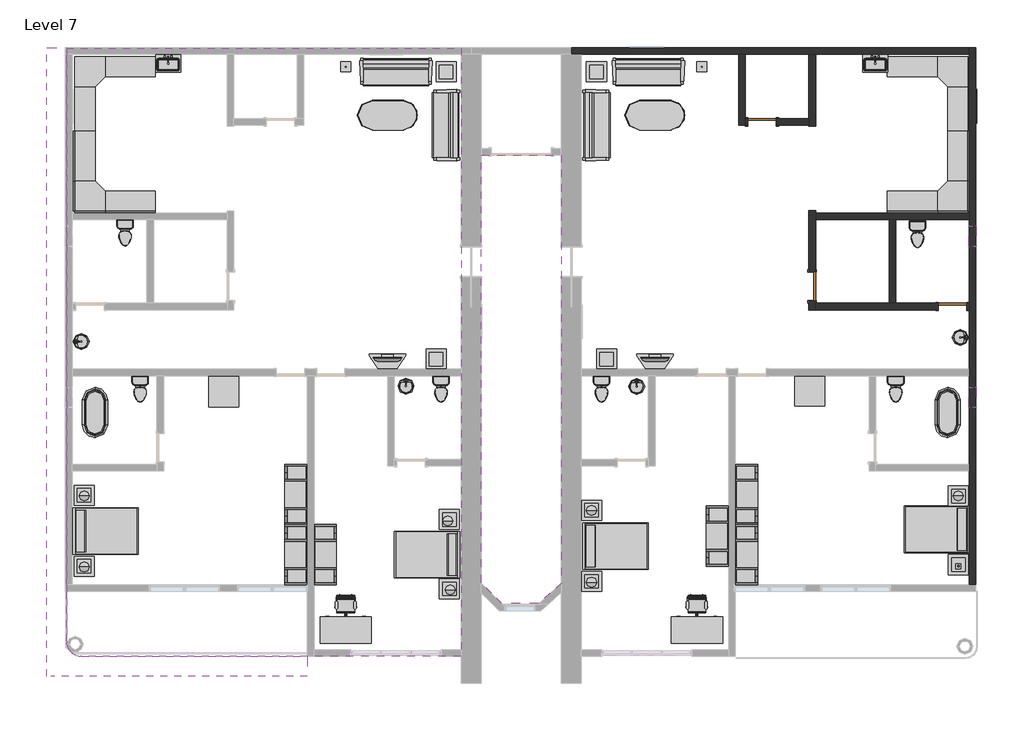
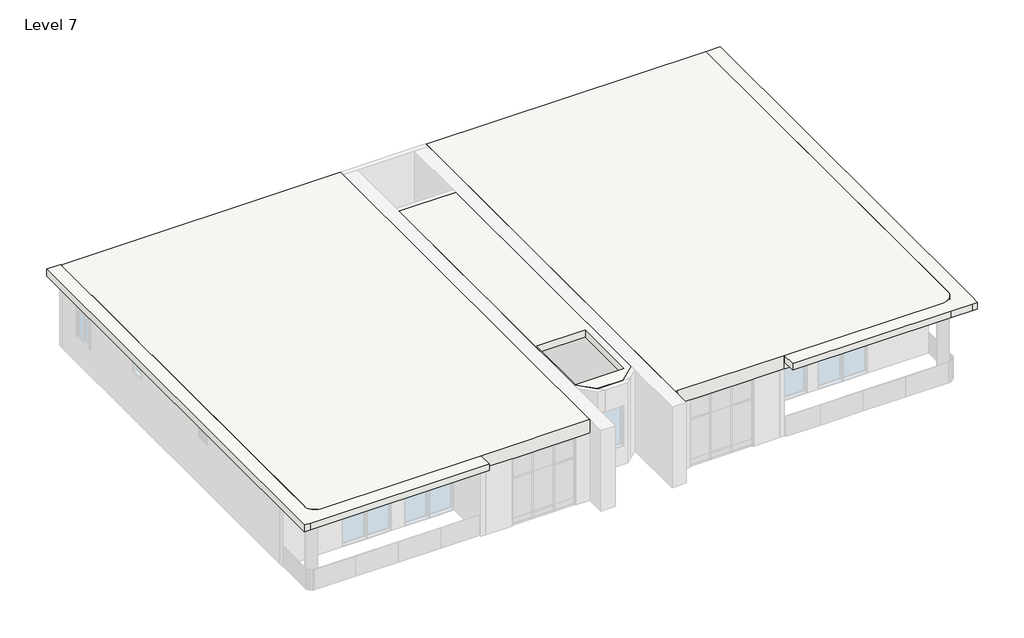
# One storey, part 3 of 3: 42 furniture elements, 14 flow terminals, 10 light fixtures, 9 walls, 3 doors, 3 slabs, 3 windows.
"""IFC4 building model written with IfcOpenShell, lengths in millimetres."""

from ifc_helpers import new_model, si_unit, point, frame, frame_2d, origin, place, context, project, spatial, polyline, circle_curve, trimmed, segment, composite_curve, outline, extrude, faceted_brep, transform, mapped, element, save
from components import door_2703ae13, door_10fd3a06, flow_terminal_38af2918, flow_terminal_d49f872f, toilet_domestic_3d_toilet_domestic_3d_f7549cf7, toilet_domestic_3d_toilet_domestic_3d_183bbd19, flow_terminal_b374fae2, furniture_07436f11, furniture_096e7f55, chair_task_arms_chair_task_arms_fa5a08ef, furniture_072f6425, furniture_cf0b6580, furniture_aff9b2fb, furniture_56245f3a, tv_stand_tv_stand_6ce107e5, furniture_b5c51a22, furniture_2c34a4f9, furniture_4d44e21c, furniture_45e3acac, light_fixture_100w_120v_8564026f, table_lamp_hemispheric_60w_120v_02721d88, window_0038ecf3, window_54100e87

model = new_model("IFC4")

# Units and contexts
model_context = context("Model", 3, world=origin())
ifc_project = project(units=[si_unit("LENGTHUNIT", "METRE", prefix="MILLI")], contexts=[model_context])

# Site, building, storey
site = spatial("IfcSite", under=ifc_project)
building = spatial("IfcBuilding", under=site)
storey = spatial("IfcBuildingStorey", under=building, Name="Level 7", Elevation=21945.6)

# Doors
placement = place(None, origin())
door_shape = door_2703ae13(model_context)
element("IfcDoor", 1, ObjectType="Door-Single-Panel.0001 : 34\" x 80\"", at=placement, inside=storey, context=model_context, shape_type="MappedRepresentation", body=[
    mapped(door_shape, transform((2528.3512296, 9464.0758558, 21945.6), x_axis=(-1.0, 0.0, 0.0), y_axis=(0.0, -1.0, 0.0), z_axis=(0.0, 0.0, 1.0))),
])
door_2_shape = door_10fd3a06(model_context)
element("IfcDoor", 2, ObjectType="Door-Single-Panel.0001 : 34\" x 80\"", at=placement, inside=storey, context=model_context, shape_type="MappedRepresentation", body=[
    mapped(door_2_shape, transform((8319.5512296, 3850.6758558, 21945.6), x_axis=(1.0, 0.0, 0.0), y_axis=(0.0, 1.0, 0.0), z_axis=(0.0, 0.0, 1.0))),
])
element("IfcDoor", 3, ObjectType="Door-Single-Panel.0001 : 34\" x 80\"", at=placement, inside=storey, context=model_context, shape_type="MappedRepresentation", body=[
    mapped(door_2_shape, transform((4052.3512296, 4460.2758558, 21945.6), x_axis=(0.0, -1.0, 0.0), y_axis=(1.0, 0.0, 0.0), z_axis=(0.0, 0.0, 1.0))),
])

# Flow terminals
flow_terminal_shape = flow_terminal_38af2918(model_context)
element("IfcFlowTerminal", 4, ObjectType="Sink Kitchen-Single : 30\" x 21\"", at=placement, inside=storey, context=model_context, shape_type="MappedRepresentation", body=[
    mapped(flow_terminal_shape, transform((-15534.038011, 11239.7304546, 21945.6), x_axis=(1.0, 0.0, 0.0), y_axis=(0.0, 1.0, 0.0), z_axis=(0.0, 0.0, 1.0))),
])
element("IfcFlowTerminal", 5, ObjectType="Sink Kitchen-Single : 30\" x 21\"", at=placement, inside=storey, context=model_context, shape_type="MappedRepresentation", body=[
    mapped(flow_terminal_shape, transform((5954.361989, 11239.7304546, 21945.6), x_axis=(1.0, 0.0, 0.0), y_axis=(0.0, 1.0, 0.0), z_axis=(0.0, 0.0, 1.0))),
])
flow_terminal_2_shape = flow_terminal_d49f872f(model_context)
element("IfcFlowTerminal", 6, ObjectType="Sink Vanity-Round : 19\" x 19\"", at=placement, inside=storey, context=model_context, shape_type="MappedRepresentation", body=[
    mapped(flow_terminal_2_shape, transform((-18078.2570794, 2687.2241152, 21945.6), x_axis=(0.0, 1.0, 0.0), y_axis=(-1.0, 0.0, 0.0), z_axis=(0.0, 0.0, 1.0))),
])
element("IfcFlowTerminal", 7, ObjectType="Sink Vanity-Round : 19\" x 19\"", at=placement, inside=storey, context=model_context, shape_type="MappedRepresentation", body=[
    mapped(flow_terminal_2_shape, transform((8468.5749463, 3007.5275963, 21945.6), x_axis=(0.0, -1.0, 0.0), y_axis=(1.0, 0.0, 0.0), z_axis=(0.0, 0.0, 1.0))),
])
element("IfcFlowTerminal", 8, ObjectType="Sink Vanity-Round : 19\" x 19\"", at=placement, inside=storey, context=model_context, shape_type="MappedRepresentation", body=[
    mapped(flow_terminal_2_shape, transform((-8388.700511, 1341.8921141, 21945.6), x_axis=(1.0, 0.0, 0.0), y_axis=(0.0, 1.0, 0.0), z_axis=(0.0, 0.0, 1.0))),
])
element("IfcFlowTerminal", 9, ObjectType="Sink Vanity-Round : 19\" x 19\"", at=placement, inside=storey, context=model_context, shape_type="MappedRepresentation", body=[
    mapped(flow_terminal_2_shape, transform((-1378.300511, 1331.0855344, 21945.6), x_axis=(1.0, 0.0, 0.0), y_axis=(0.0, 1.0, 0.0), z_axis=(0.0, 0.0, 1.0))),
])
toilet_domestic_3d_toilet_domestic_3d_shape = toilet_domestic_3d_toilet_domestic_3d_f7549cf7(model_context)
toilet_domestic_3d_toilet_domestic_3d_2_shape = toilet_domestic_3d_toilet_domestic_3d_183bbd19(model_context)
element("IfcFlowTerminal", 10, ObjectType="Toilet-Domestic-3D : Toilet-Domestic-3D", at=placement, inside=storey, context=model_context, shape_type="MappedRepresentation", body=[
    mapped(toilet_domestic_3d_toilet_domestic_3d_shape, transform((6592.3512296, 1247.7798284, 21945.6), x_axis=(1.0, 0.0, 0.0), y_axis=(0.0, 1.0, 0.0), z_axis=(0.0, 0.0, 1.0))),
    mapped(toilet_domestic_3d_toilet_domestic_3d_2_shape, transform((6592.3512296, 1247.7798284, 21945.6), x_axis=(1.0, 0.0, 0.0), y_axis=(0.0, 1.0, 0.0), z_axis=(0.0, 0.0, 1.0))),
])
element("IfcFlowTerminal", 11, ObjectType="Toilet-Domestic-3D : Toilet-Domestic-3D", at=placement, inside=storey, context=model_context, shape_type="MappedRepresentation", body=[
    mapped(toilet_domestic_3d_toilet_domestic_3d_shape, transform((-2348.4487704, 1247.7798284, 21945.6), x_axis=(1.0, 0.0, 0.0), y_axis=(0.0, 1.0, 0.0), z_axis=(0.0, 0.0, 1.0))),
    mapped(toilet_domestic_3d_toilet_domestic_3d_2_shape, transform((-2348.4487704, 1247.7798284, 21945.6), x_axis=(1.0, 0.0, 0.0), y_axis=(0.0, 1.0, 0.0), z_axis=(0.0, 0.0, 1.0))),
])
element("IfcFlowTerminal", 12, ObjectType="Toilet-Domestic-3D : Toilet-Domestic-3D", at=placement, inside=storey, context=model_context, shape_type="MappedRepresentation", body=[
    mapped(toilet_domestic_3d_toilet_domestic_3d_shape, transform((-16369.2487704, 1247.7798284, 21945.6), x_axis=(1.0, 0.0, 0.0), y_axis=(0.0, 1.0, 0.0), z_axis=(0.0, 0.0, 1.0))),
    mapped(toilet_domestic_3d_toilet_domestic_3d_2_shape, transform((-16369.2487704, 1247.7798284, 21945.6), x_axis=(1.0, 0.0, 0.0), y_axis=(0.0, 1.0, 0.0), z_axis=(0.0, 0.0, 1.0))),
])
element("IfcFlowTerminal", 13, ObjectType="Toilet-Domestic-3D : Toilet-Domestic-3D", at=placement, inside=storey, context=model_context, shape_type="MappedRepresentation", body=[
    mapped(toilet_domestic_3d_toilet_domestic_3d_shape, transform((-16826.4487704, 5997.5798284, 21945.6), x_axis=(1.0, 0.0, 0.0), y_axis=(0.0, 1.0, 0.0), z_axis=(0.0, 0.0, 1.0))),
    mapped(toilet_domestic_3d_toilet_domestic_3d_2_shape, transform((-16826.4487704, 5997.5798284, 21945.6), x_axis=(1.0, 0.0, 0.0), y_axis=(0.0, 1.0, 0.0), z_axis=(0.0, 0.0, 1.0))),
])
element("IfcFlowTerminal", 14, ObjectType="Toilet-Domestic-3D : Toilet-Domestic-3D", at=placement, inside=storey, context=model_context, shape_type="MappedRepresentation", body=[
    mapped(toilet_domestic_3d_toilet_domestic_3d_shape, transform((7252.7512296, 5946.7798284, 21945.6), x_axis=(1.0, 0.0, 0.0), y_axis=(0.0, 1.0, 0.0), z_axis=(0.0, 0.0, 1.0))),
    mapped(toilet_domestic_3d_toilet_domestic_3d_2_shape, transform((7252.7512296, 5946.7798284, 21945.6), x_axis=(1.0, 0.0, 0.0), y_axis=(0.0, 1.0, 0.0), z_axis=(0.0, 0.0, 1.0))),
])
element("IfcFlowTerminal", 15, ObjectType="Toilet-Domestic-3D : Toilet-Domestic-3D", at=placement, inside=storey, context=model_context, shape_type="MappedRepresentation", body=[
    mapped(toilet_domestic_3d_toilet_domestic_3d_shape, transform((-7225.2487704, 1247.7798284, 21945.6), x_axis=(1.0, 0.0, 0.0), y_axis=(0.0, 1.0, 0.0), z_axis=(0.0, 0.0, 1.0))),
    mapped(toilet_domestic_3d_toilet_domestic_3d_2_shape, transform((-7225.2487704, 1247.7798284, 21945.6), x_axis=(1.0, 0.0, 0.0), y_axis=(0.0, 1.0, 0.0), z_axis=(0.0, 0.0, 1.0))),
])
flow_terminal_3_shape = flow_terminal_b374fae2(model_context)
element("IfcFlowTerminal", 16, ObjectType="Tub-Free Standing-3D : 30\" x 60\"", at=placement, inside=storey, context=model_context, shape_type="MappedRepresentation", body=[
    mapped(flow_terminal_3_shape, transform((-17740.8487704, 624.8758558, 21945.6), x_axis=(1.0, 0.0, 0.0), y_axis=(0.0, 1.0, 0.0), z_axis=(0.0, 0.0, 1.0))),
])
element("IfcFlowTerminal", 17, ObjectType="Tub-Free Standing-3D : 30\" x 60\"", at=placement, inside=storey, context=model_context, shape_type="MappedRepresentation", body=[
    mapped(flow_terminal_3_shape, transform((8167.1512296, 624.8758558, 21945.6), x_axis=(1.0, 0.0, 0.0), y_axis=(0.0, 1.0, 0.0), z_axis=(0.0, 0.0, 1.0))),
])

# Furniture
furniture_shape = furniture_07436f11(model_context)
element("IfcFurniture", 18, ObjectType="96\" x 96\"", at=placement, inside=storey, context=model_context, shape_type="MappedRepresentation", body=[
    mapped(furniture_shape, transform((-18269.5170182, 11991.0988634, 21945.6), x_axis=(1.0, 0.0, 0.0), y_axis=(0.0, 1.0, 0.0), z_axis=(0.0, 0.0, 1.0))),
])
element("IfcFurniture", 19, ObjectType="96\" x 96\"", at=placement, inside=storey, context=model_context, shape_type="MappedRepresentation", body=[
    mapped(furniture_shape, transform((9322.5742372, 11364.3441035, 21945.6), x_axis=(0.0, -1.0, 0.0), y_axis=(1.0, 0.0, 0.0), z_axis=(0.0, 0.0, 1.0))),
])
furniture_2_shape = furniture_096e7f55(model_context)
element("IfcFurniture", 20, ObjectType="Bed-Shaker : Double 56\" x 78\"", at=placement, inside=storey, context=model_context, shape_type="MappedRepresentation", body=[
    mapped(furniture_2_shape, transform((-18401.2487704, -2962.8741442, 21945.6), x_axis=(0.0, 1.0, 0.0), y_axis=(-1.0, 0.0, 0.0), z_axis=(0.0, 0.0, 1.0))),
])
element("IfcFurniture", 21, ObjectType="Bed-Shaker : Double 56\" x 78\"", at=placement, inside=storey, context=model_context, shape_type="MappedRepresentation", body=[
    mapped(furniture_2_shape, transform((-6666.4487704, -3712.1741442, 21945.6), x_axis=(0.0, -1.0, 0.0), y_axis=(1.0, 0.0, 0.0), z_axis=(0.0, 0.0, 1.0))),
])
element("IfcFurniture", 22, ObjectType="Bed-Shaker : Double 56\" x 78\"", at=placement, inside=storey, context=model_context, shape_type="MappedRepresentation", body=[
    mapped(furniture_2_shape, transform((-2907.2487704, -3420.0741442, 21945.6), x_axis=(0.0, 1.0, 0.0), y_axis=(-1.0, 0.0, 0.0), z_axis=(0.0, 0.0, 1.0))),
])
element("IfcFurniture", 23, ObjectType="Bed-Shaker : Double 56\" x 78\"", at=placement, inside=storey, context=model_context, shape_type="MappedRepresentation", body=[
    mapped(furniture_2_shape, transform((8827.5512296, -2950.1741442, 21945.6), x_axis=(0.0, -1.0, 0.0), y_axis=(1.0, 0.0, 0.0), z_axis=(0.0, 0.0, 1.0))),
])
chair_task_arms_chair_task_arms_shape = chair_task_arms_chair_task_arms_fa5a08ef(model_context)
element("IfcFurniture", 24, ObjectType="Chair-Task Arms : Chair-Task Arms", at=placement, inside=storey, context=model_context, shape_type="MappedRepresentation", body=[
    mapped(chair_task_arms_chair_task_arms_shape, transform((688.1420493, -5184.3566833, 21945.6), x_axis=(-1.0, 0.0, 0.0), y_axis=(0.0, -1.0, 0.0), z_axis=(0.0, 0.0, 1.0))),
])
element("IfcFurniture", 25, ObjectType="Chair-Task Arms : Chair-Task Arms", at=placement, inside=storey, context=model_context, shape_type="MappedRepresentation", body=[
    mapped(chair_task_arms_chair_task_arms_shape, transform((-9979.8579507, -5184.3566833, 21945.6), x_axis=(-1.0, 0.0, 0.0), y_axis=(0.0, -1.0, 0.0), z_axis=(0.0, 0.0, 1.0))),
])
furniture_3_shape = furniture_072f6425(model_context)
element("IfcFurniture", 26, ObjectType="Desk : 60\" x 30\"", at=placement, inside=storey, context=model_context, shape_type="MappedRepresentation", body=[
    mapped(furniture_3_shape, transform((-10882.8487704, -6371.702585, 21945.6), x_axis=(1.0, 0.0, 0.0), y_axis=(0.0, 1.0, 0.0), z_axis=(0.0, 0.0, 1.0))),
])
element("IfcFurniture", 27, ObjectType="Desk : 60\" x 30\"", at=placement, inside=storey, context=model_context, shape_type="MappedRepresentation", body=[
    mapped(furniture_3_shape, transform((-214.8487704, -6371.702585, 21945.6), x_axis=(1.0, 0.0, 0.0), y_axis=(0.0, 1.0, 0.0), z_axis=(0.0, 0.0, 1.0))),
])
furniture_4_shape = furniture_cf0b6580(model_context)
element("IfcFurniture", 28, ObjectType="Entertainment Center : 72\" x 72\" x 24\"", at=placement, inside=storey, context=model_context, shape_type="MappedRepresentation", body=[
    mapped(furniture_4_shape, transform((1613.9512296, -3134.3241442, 21945.6), x_axis=(0.0, -1.0, 0.0), y_axis=(1.0, 0.0, 0.0), z_axis=(0.0, 0.0, 1.0))),
])
element("IfcFurniture", 29, ObjectType="Entertainment Center : 72\" x 72\" x 24\"", at=placement, inside=storey, context=model_context, shape_type="MappedRepresentation", body=[
    mapped(furniture_4_shape, transform((1613.9512296, -3693.1241442, 21945.6), x_axis=(0.0, 1.0, 0.0), y_axis=(-1.0, 0.0, 0.0), z_axis=(0.0, 0.0, 1.0))),
])
element("IfcFurniture", 30, ObjectType="Entertainment Center : 72\" x 72\" x 24\"", at=placement, inside=storey, context=model_context, shape_type="MappedRepresentation", body=[
    mapped(furniture_4_shape, transform((1613.9512296, -1864.3241442, 21945.6), x_axis=(0.0, 1.0, 0.0), y_axis=(-1.0, 0.0, 0.0), z_axis=(0.0, 0.0, 1.0))),
])
element("IfcFurniture", 31, ObjectType="Entertainment Center : 72\" x 72\" x 24\"", at=placement, inside=storey, context=model_context, shape_type="MappedRepresentation", body=[
    mapped(furniture_4_shape, transform((-11187.6487704, -3693.1241442, 21945.6), x_axis=(0.0, -1.0, 0.0), y_axis=(1.0, 0.0, 0.0), z_axis=(0.0, 0.0, 1.0))),
])
element("IfcFurniture", 32, ObjectType="Entertainment Center : 72\" x 72\" x 24\"", at=placement, inside=storey, context=model_context, shape_type="MappedRepresentation", body=[
    mapped(furniture_4_shape, transform((-11187.6487704, -1864.3241442, 21945.6), x_axis=(0.0, -1.0, 0.0), y_axis=(1.0, 0.0, 0.0), z_axis=(0.0, 0.0, 1.0))),
])
element("IfcFurniture", 33, ObjectType="Entertainment Center : 72\" x 72\" x 24\"", at=placement, inside=storey, context=model_context, shape_type="MappedRepresentation", body=[
    mapped(furniture_4_shape, transform((-11187.6487704, -3693.1241442, 21945.6), x_axis=(0.0, 1.0, 0.0), y_axis=(-1.0, 0.0, 0.0), z_axis=(0.0, 0.0, 1.0))),
])
furniture_5_shape = furniture_aff9b2fb(model_context)
element("IfcFurniture", 34, ObjectType="Sofa-Pensi : 84\"", at=placement, inside=storey, context=model_context, shape_type="MappedRepresentation", body=[
    mapped(furniture_5_shape, transform((-8875.4550204, 10710.9660197, 21945.6), x_axis=(1.0, 0.0, 0.0), y_axis=(0.0, 1.0, 0.0), z_axis=(0.0, 0.0, 1.0))),
])
element("IfcFurniture", 35, ObjectType="Sofa-Pensi : 84\"", at=placement, inside=storey, context=model_context, shape_type="MappedRepresentation", body=[
    mapped(furniture_5_shape, transform((-7349.9586065, 9641.0821058, 21945.6), x_axis=(0.0, -1.0, 0.0), y_axis=(1.0, 0.0, 0.0), z_axis=(0.0, 0.0, 1.0))),
])
element("IfcFurniture", 36, ObjectType="Sofa-Pensi : 84\"", at=placement, inside=storey, context=model_context, shape_type="MappedRepresentation", body=[
    mapped(furniture_5_shape, transform((-2223.7389343, 9083.8696058, 21945.6), x_axis=(0.0, 1.0, 0.0), y_axis=(-1.0, 0.0, 0.0), z_axis=(0.0, 0.0, 1.0))),
])
element("IfcFurniture", 37, ObjectType="Sofa-Pensi : 84\"", at=placement, inside=storey, context=model_context, shape_type="MappedRepresentation", body=[
    mapped(furniture_5_shape, transform((-1204.6550204, 10710.9660197, 21945.6), x_axis=(1.0, 0.0, 0.0), y_axis=(0.0, 1.0, 0.0), z_axis=(0.0, 0.0, 1.0))),
])
furniture_6_shape = furniture_56245f3a(model_context)
element("IfcFurniture", 38, ObjectType="TV - Flat Screen : 32\"", at=placement, inside=storey, context=model_context, shape_type="MappedRepresentation", body=[
    mapped(furniture_6_shape, transform((-8854.7932846, 2232.8144794, 22860.0), x_axis=(-1.0, 0.0, 0.0), y_axis=(0.0, -1.0, 0.0), z_axis=(0.0, 0.0, 1.0))),
])
element("IfcFurniture", 39, ObjectType="TV - Flat Screen : 32\"", at=placement, inside=storey, context=model_context, shape_type="MappedRepresentation", body=[
    mapped(furniture_6_shape, transform((-726.7932846, 2232.8144794, 22860.0), x_axis=(-1.0, 0.0, 0.0), y_axis=(0.0, -1.0, 0.0), z_axis=(0.0, 0.0, 1.0))),
])
tv_stand_tv_stand_shape = tv_stand_tv_stand_6ce107e5(model_context)
element("IfcFurniture", 40, ObjectType="TV Stand : TV Stand", at=placement, inside=storey, context=model_context, shape_type="MappedRepresentation", body=[
    mapped(tv_stand_tv_stand_shape, transform((-8725.6607683, 1945.6758558, 21945.6), x_axis=(-1.0, 0.0, 0.0), y_axis=(0.0, -1.0, 0.0), z_axis=(0.0, 0.0, 1.0))),
])
element("IfcFurniture", 41, ObjectType="TV Stand : TV Stand", at=placement, inside=storey, context=model_context, shape_type="MappedRepresentation", body=[
    mapped(tv_stand_tv_stand_shape, transform((-597.6607683, 1945.6758558, 21945.6), x_axis=(-1.0, 0.0, 0.0), y_axis=(0.0, -1.0, 0.0), z_axis=(0.0, 0.0, 1.0))),
])
furniture_7_shape = furniture_b5c51a22(model_context)
element("IfcFurniture", 42, ObjectType="Table-Coffee : 24\" x 24\" x 24\"", at=placement, inside=storey, context=model_context, shape_type="MappedRepresentation", body=[
    mapped(furniture_7_shape, transform((-7091.1145371, 10892.864778, 21945.6), x_axis=(1.0, 0.0, 0.0), y_axis=(0.0, 1.0, 0.0), z_axis=(0.0, 0.0, 1.0))),
])
element("IfcFurniture", 43, ObjectType="Table-Coffee : 24\" x 24\" x 24\"", at=placement, inside=storey, context=model_context, shape_type="MappedRepresentation", body=[
    mapped(furniture_7_shape, transform((-2519.1145371, 10892.864778, 21945.6), x_axis=(1.0, 0.0, 0.0), y_axis=(0.0, 1.0, 0.0), z_axis=(0.0, 0.0, 1.0))),
])
element("IfcFurniture", 44, ObjectType="Table-Coffee : 24\" x 24\" x 24\"", at=placement, inside=storey, context=model_context, shape_type="MappedRepresentation", body=[
    mapped(furniture_7_shape, transform((-7395.9145371, 2155.264778, 21945.6), x_axis=(1.0, 0.0, 0.0), y_axis=(0.0, 1.0, 0.0), z_axis=(0.0, 0.0, 1.0))),
])
element("IfcFurniture", 45, ObjectType="Table-Coffee : 24\" x 24\" x 24\"", at=placement, inside=storey, context=model_context, shape_type="MappedRepresentation", body=[
    mapped(furniture_7_shape, transform((-2214.3145371, 2155.264778, 21945.6), x_axis=(1.0, 0.0, 0.0), y_axis=(0.0, 1.0, 0.0), z_axis=(0.0, 0.0, 1.0))),
])
element("IfcFurniture", 46, ObjectType="Table-Coffee : 24\" x 24\" x 24\"", at=placement, inside=storey, context=model_context, shape_type="MappedRepresentation", body=[
    mapped(furniture_7_shape, transform((-2671.5145371, -4601.135222, 21945.6), x_axis=(1.0, 0.0, 0.0), y_axis=(0.0, 1.0, 0.0), z_axis=(0.0, 0.0, 1.0))),
])
element("IfcFurniture", 47, ObjectType="Table-Coffee : 24\" x 24\" x 24\"", at=placement, inside=storey, context=model_context, shape_type="MappedRepresentation", body=[
    mapped(furniture_7_shape, transform((-18089.3145371, -4143.935222, 21945.6), x_axis=(1.0, 0.0, 0.0), y_axis=(0.0, 1.0, 0.0), z_axis=(0.0, 0.0, 1.0))),
])
element("IfcFurniture", 48, ObjectType="Table-Coffee : 24\" x 24\" x 24\"", at=placement, inside=storey, context=model_context, shape_type="MappedRepresentation", body=[
    mapped(furniture_7_shape, transform((-18089.3145371, -1984.935222, 21945.6), x_axis=(1.0, 0.0, 0.0), y_axis=(0.0, 1.0, 0.0), z_axis=(0.0, 0.0, 1.0))),
])
element("IfcFurniture", 49, ObjectType="Table-Coffee : 24\" x 24\" x 24\"", at=placement, inside=storey, context=model_context, shape_type="MappedRepresentation", body=[
    mapped(furniture_7_shape, transform((-2671.5145371, -2442.135222, 21945.6), x_axis=(1.0, 0.0, 0.0), y_axis=(0.0, 1.0, 0.0), z_axis=(0.0, 0.0, 1.0))),
])
element("IfcFurniture", 50, ObjectType="Table-Coffee : 24\" x 24\" x 24\"", at=placement, inside=storey, context=model_context, shape_type="MappedRepresentation", body=[
    mapped(furniture_7_shape, transform((8479.0854629, -4093.135222, 21945.6), x_axis=(1.0, 0.0, 0.0), y_axis=(0.0, 1.0, 0.0), z_axis=(0.0, 0.0, 1.0))),
])
element("IfcFurniture", 51, ObjectType="Table-Coffee : 24\" x 24\" x 24\"", at=placement, inside=storey, context=model_context, shape_type="MappedRepresentation", body=[
    mapped(furniture_7_shape, transform((8479.0854629, -2010.335222, 21945.6), x_axis=(1.0, 0.0, 0.0), y_axis=(0.0, 1.0, 0.0), z_axis=(0.0, 0.0, 1.0))),
])
element("IfcFurniture", 52, ObjectType="Table-Coffee : 24\" x 24\" x 24\"", at=placement, inside=storey, context=model_context, shape_type="MappedRepresentation", body=[
    mapped(furniture_7_shape, transform((-6989.5145371, -4832.0414601, 21945.6), x_axis=(1.0, 0.0, 0.0), y_axis=(0.0, 1.0, 0.0), z_axis=(0.0, 0.0, 1.0))),
])
element("IfcFurniture", 53, ObjectType="Table-Coffee : 24\" x 24\" x 24\"", at=placement, inside=storey, context=model_context, shape_type="MappedRepresentation", body=[
    mapped(furniture_7_shape, transform((-6989.5145371, -2723.8414601, 21945.6), x_axis=(1.0, 0.0, 0.0), y_axis=(0.0, 1.0, 0.0), z_axis=(0.0, 0.0, 1.0))),
])
furniture_8_shape = furniture_2c34a4f9(model_context)
element("IfcFurniture", 54, ObjectType="Table-Dining Oval : 36\" x 72\"", at=placement, inside=storey, context=model_context, shape_type="MappedRepresentation", body=[
    mapped(furniture_8_shape, transform((-8449.0290983, 10025.3742164, 21945.6), x_axis=(1.0, 0.0, 0.0), y_axis=(0.0, 1.0, 0.0), z_axis=(0.0, 0.0, 1.0))),
])
element("IfcFurniture", 55, ObjectType="Table-Dining Oval : 36\" x 72\"", at=placement, inside=storey, context=model_context, shape_type="MappedRepresentation", body=[
    mapped(furniture_8_shape, transform((-321.0290983, 10025.3742164, 21945.6), x_axis=(1.0, 0.0, 0.0), y_axis=(0.0, 1.0, 0.0), z_axis=(0.0, 0.0, 1.0))),
])
furniture_9_shape = furniture_4d44e21c(model_context)
element("IfcFurniture", 56, ObjectType="Table-Rectangular : 36\" x 36\"", at=placement, inside=storey, context=model_context, shape_type="MappedRepresentation", body=[
    mapped(furniture_9_shape, transform((-13829.2487704, 1259.8758558, 21945.6), x_axis=(1.0, 0.0, 0.0), y_axis=(0.0, 1.0, 0.0), z_axis=(0.0, 0.0, 1.0))),
])
element("IfcFurniture", 57, ObjectType="Table-Rectangular : 36\" x 36\"", at=placement, inside=storey, context=model_context, shape_type="MappedRepresentation", body=[
    mapped(furniture_9_shape, transform((3976.1512296, 1285.2758558, 21945.6), x_axis=(1.0, 0.0, 0.0), y_axis=(0.0, 1.0, 0.0), z_axis=(0.0, 0.0, 1.0))),
])
furniture_10_shape = furniture_45e3acac(model_context)
element("IfcFurniture", 58, ObjectType="Work Station Cubicle : 96\" x 96\"", at=placement, inside=storey, context=model_context, shape_type="MappedRepresentation", body=[
    mapped(furniture_10_shape, transform((-18896.271778, 6827.207608, 21945.6), x_axis=(0.0, 1.0, 0.0), y_axis=(-1.0, 0.0, 0.0), z_axis=(0.0, 0.0, 1.0))),
])
element("IfcFurniture", 59, ObjectType="Work Station Cubicle : 96\" x 96\"", at=placement, inside=storey, context=model_context, shape_type="MappedRepresentation", body=[
    mapped(furniture_10_shape, transform((8695.8194774, 6200.4528481, 21945.6), x_axis=(-1.0, 0.0, 0.0), y_axis=(0.0, -1.0, 0.0), z_axis=(0.0, 0.0, 1.0))),
])

# Light fixtures
light_fixture_100w_120v_shape = light_fixture_100w_120v_8564026f(model_context)
element("IfcLightFixture", 60, ObjectType="100W - 120V", at=placement, inside=storey, context=model_context, shape_type="MappedRepresentation", body=[
    mapped(light_fixture_100w_120v_shape, transform((-10120.8487704, 11140.4758558, 21945.6), x_axis=(1.0, 0.0, 0.0), y_axis=(0.0, 1.0, 0.0), z_axis=(0.0, 0.0, 1.0))),
])
element("IfcLightFixture", 61, ObjectType="100W - 120V", at=placement, inside=storey, context=model_context, shape_type="MappedRepresentation", body=[
    mapped(light_fixture_100w_120v_shape, transform((699.5512296, 11140.4758558, 21945.6), x_axis=(1.0, 0.0, 0.0), y_axis=(0.0, 1.0, 0.0), z_axis=(0.0, 0.0, 1.0))),
])
table_lamp_hemispheric_60w_120v_shape = table_lamp_hemispheric_60w_120v_02721d88(model_context)
element("IfcLightFixture", 62, ObjectType="Table Lamp - Hemispheric : 60W - 120V", at=placement, inside=storey, context=model_context, shape_type="MappedRepresentation", body=[
    mapped(table_lamp_hemispheric_60w_120v_shape, transform((-18071.0487704, -1915.1241442, 22555.2), x_axis=(1.0, 0.0, 0.0), y_axis=(0.0, 1.0, 0.0), z_axis=(0.0, 0.0, 1.0))),
])
element("IfcLightFixture", 63, ObjectType="Table Lamp - Hemispheric : 60W - 120V", at=placement, inside=storey, context=model_context, shape_type="MappedRepresentation", body=[
    mapped(table_lamp_hemispheric_60w_120v_shape, transform((-7022.0487704, -2666.7303823, 22555.2), x_axis=(1.0, 0.0, 0.0), y_axis=(0.0, 1.0, 0.0), z_axis=(0.0, 0.0, 1.0))),
])
element("IfcLightFixture", 64, ObjectType="Table Lamp - Hemispheric : 60W - 120V", at=placement, inside=storey, context=model_context, shape_type="MappedRepresentation", body=[
    mapped(table_lamp_hemispheric_60w_120v_shape, transform((-2653.2487704, -2346.9241442, 22555.2), x_axis=(1.0, 0.0, 0.0), y_axis=(0.0, 1.0, 0.0), z_axis=(0.0, 0.0, 1.0))),
])
element("IfcLightFixture", 65, ObjectType="Table Lamp - Hemispheric : 60W - 120V", at=placement, inside=storey, context=model_context, shape_type="MappedRepresentation", body=[
    mapped(table_lamp_hemispheric_60w_120v_shape, transform((8497.3512296, -4048.7241442, 22860.0), x_axis=(1.0, 0.0, 0.0), y_axis=(0.0, 1.0, 0.0), z_axis=(0.0, 0.0, 1.0))),
])
element("IfcLightFixture", 66, ObjectType="Table Lamp - Hemispheric : 60W - 120V", at=placement, inside=storey, context=model_context, shape_type="MappedRepresentation", body=[
    mapped(table_lamp_hemispheric_60w_120v_shape, transform((8497.3512296, -1915.1241442, 22555.2), x_axis=(1.0, 0.0, 0.0), y_axis=(0.0, 1.0, 0.0), z_axis=(0.0, 0.0, 1.0))),
])
element("IfcLightFixture", 67, ObjectType="Table Lamp - Hemispheric : 60W - 120V", at=placement, inside=storey, context=model_context, shape_type="MappedRepresentation", body=[
    mapped(table_lamp_hemispheric_60w_120v_shape, transform((-2653.2487704, -4531.3241442, 22555.2), x_axis=(1.0, 0.0, 0.0), y_axis=(0.0, 1.0, 0.0), z_axis=(0.0, 0.0, 1.0))),
])
element("IfcLightFixture", 68, ObjectType="Table Lamp - Hemispheric : 60W - 120V", at=placement, inside=storey, context=model_context, shape_type="MappedRepresentation", body=[
    mapped(table_lamp_hemispheric_60w_120v_shape, transform((-6945.8487704, -4762.2303823, 22555.2), x_axis=(1.0, 0.0, 0.0), y_axis=(0.0, 1.0, 0.0), z_axis=(0.0, 0.0, 1.0))),
])
element("IfcLightFixture", 69, ObjectType="Table Lamp - Hemispheric : 60W - 120V", at=placement, inside=storey, context=model_context, shape_type="MappedRepresentation", body=[
    mapped(table_lamp_hemispheric_60w_120v_shape, transform((-18071.0487704, -4074.1241442, 22555.2), x_axis=(1.0, 0.0, 0.0), y_axis=(0.0, 1.0, 0.0), z_axis=(0.0, 0.0, 1.0))),
])

# Slabs
element("IfcSlab", 70, ObjectType="Generic - 12\" cream", at=placement, inside=storey, context=model_context, shape_type="SweptSolid", body=[
    extrude(outline(composite_curve([segment(polyline([(-6615.6487704, 11699.2758558), (-6615.6487704, -6791.9241442), (-11289.2487704, -6791.9241442), (-18147.2487704, -6791.9241442)]), True, "CONTINUOUS"), segment(trimmed(circle_curve(frame_2d((-18147.2487704, -6334.7241442)), 457.2), [point((-18147.2487704, -6791.9241442))], [point((-18604.4487704, -6334.7241442))], False, "CARTESIAN"), True, "CONTINUOUS"), segment(polyline([(-18604.4487704, -6334.7241442), (-18604.4487704, 11699.2758558), (-6615.6487704, 11699.2758558)]), True, "CONTINUOUS")], self_intersect=False)), frame((0.0, 0.0, 24993.6), z_axis=(0.0, 0.0, 1.0), x_axis=(1.0, 0.0, 0.0)), (0.0, 0.0, 1.0), 609.6),
    extrude(outline(composite_curve([segment(trimmed(circle_curve(frame_2d((8518.1543381, -6277.3874522)), 514.536692), [point((9030.7512296, -6322.0241442))], [point((8518.1543381, -6791.9241442))], False, "CARTESIAN"), True, "CONTINUOUS"), segment(polyline([(8518.1543381, -6791.9241442), (1715.5512296, -6791.9241442), (-2856.4487704, -6791.9241442), (-2958.0487704, -6791.9241442), (-2958.0487704, 11699.2758558), (9030.7512296, 11699.2758558), (9030.7512296, -6322.0241442)]), True, "CONTINUOUS")], self_intersect=False)), frame((0.0, 0.0, 24993.6), z_axis=(0.0, 0.0, 1.0), x_axis=(1.0, 0.0, 0.0)), (0.0, 0.0, 1.0), 609.6),
])
element("IfcSlab", 71, ObjectType="Generic - 12\" white", at=placement, inside=storey, context=model_context, shape_type="SweptSolid", body=[
    extrude(outline(composite_curve([segment(polyline([(9640.3512296, 11699.2758558), (9640.3512296, -6931.6241442), (9640.3512296, -7401.5241442), (9437.1512296, -7401.5241442), (8518.1543381, -7401.5241442), (1715.5512296, -7401.5241442), (1715.5512296, -6791.9241442), (8518.1543381, -6791.9241442)]), True, "CONTINUOUS"), segment(trimmed(circle_curve(frame_2d((8518.1543381, -6277.3874522)), 514.536692), [point((8518.1543381, -6791.9241442))], [point((9030.7512296, -6322.0241442))], True, "CARTESIAN"), True, "CONTINUOUS"), segment(polyline([(9030.7512296, -6322.0241442), (9030.7512296, 11699.2758558), (9640.3512296, 11699.2758558)]), True, "CONTINUOUS")], self_intersect=False)), frame((0.0, 0.0, 25298.4), z_axis=(0.0, 0.0, 1.0), x_axis=(1.0, 0.0, 0.0)), (0.0, 0.0, 1.0), 304.8),
    extrude(outline(composite_curve([segment(polyline([(-18604.4487704, 11724.6758558), (-18604.4487704, -6334.7241442)]), True, "CONTINUOUS"), segment(trimmed(circle_curve(frame_2d((-18147.2487704, -6334.7241442)), 457.2), [point((-18604.4487704, -6334.7241442))], [point((-18147.2487704, -6791.9241442))], True, "CARTESIAN"), True, "CONTINUOUS"), segment(polyline([(-18147.2487704, -6791.9241442), (-11289.2487704, -6791.9241442), (-11289.2487704, -7401.5241442), (-18960.0487704, -7401.5241442), (-19214.0487704, -7401.5241442), (-19214.0487704, 11724.6758558), (-18604.4487704, 11724.6758558)]), True, "CONTINUOUS")], self_intersect=False)), frame((0.0, 0.0, 25298.4), z_axis=(0.0, 0.0, 1.0), x_axis=(1.0, 0.0, 0.0)), (0.0, 0.0, 1.0), 304.8),
])
element("IfcSlab", 72, ObjectType="Generic - 12\" white", at=placement, inside=storey, context=model_context, shape_type="SweptSolid", body=[
    extrude(outline(polyline([(-3573.9987704, 8448.0758558), (-3573.9987704, -1691.5549149), (-3573.9987704, -4572.9908503), (-4256.4404958, -5181.5963477), (-5374.0404958, -5181.5963477), (-6006.0487704, -4549.5880731), (-6006.0487704, -1691.5549149), (-6006.0487704, 8448.0758558), (-3573.9987704, 8448.0758558)]), holes=[polyline([(-5940.8822214, -4561.7549149), (-3870.7822214, -4561.7549149), (-3870.7822214, -1691.5549149), (-5940.8822214, -1691.5549149), (-5940.8822214, -4561.7549149)])]), frame((0.0, 0.0, 25298.4), z_axis=(0.0, 0.0, 1.0), x_axis=(1.0, 0.0, 0.0)), (0.0, 0.0, 1.0), 304.8),
])

# Walls
element("IfcWall", 73, ObjectType="Generic - 8\" cream", at=placement, inside=storey, context=model_context, shape_type="Brep", body=[
    faceted_brep([(8827.5512296, 11724.6758558, 21945.6), (8827.5512296, 11521.4758558, 21945.6), (8827.5512296, 6695.4758558, 21945.6), (8827.5512296, 6492.2758558, 21945.6), (8827.5512296, 3952.2758558, 21945.6), (8827.5512296, 3749.0758558, 21945.6), (8827.5512296, 1945.6758558, 21945.6), (8827.5512296, 1742.4758558, 21945.6), (8827.5512296, -949.9241442, 21945.6), (8827.5512296, -1153.1241442, 21945.6), (8827.5512296, -4607.5241442, 21945.6), (8827.5512296, -4607.5241442, 24993.6), (8827.5512296, -1153.1241442, 24993.6), (8827.5512296, -949.9241442, 24993.6), (8827.5512296, 1742.4758558, 24993.6), (8827.5512296, 1945.6758558, 24993.6), (8827.5512296, 3749.0758558, 24993.6), (8827.5512296, 3952.2758558, 24993.6), (8827.5512296, 6492.2758558, 24993.6), (8827.5512296, 6695.4758558, 24993.6), (8827.5512296, 11521.4758558, 24993.6), (8827.5512296, 11724.6758558, 24993.6), (8827.5512296, 10403.8758558, 23164.8), (8827.5512296, 10403.8758558, 24384.0), (8827.5512296, 9489.4758558, 24384.0), (8827.5512296, 9489.4758558, 23164.8), (8827.5512296, 777.2758558, 24688.8), (8827.5512296, 777.2758558, 24079.2), (8827.5512296, 1386.8758558, 24079.2), (8827.5512296, 1386.8758558, 24688.8), (8827.5512296, 6289.0758558, 24079.2), (8827.5512296, 6289.0758558, 24688.8), (8827.5512296, 5679.4758558, 24688.8), (8827.5512296, 5679.4758558, 24079.2), (9030.7512296, -4607.5241442, 21945.6), (9030.7512296, 11724.6758558, 21945.6), (9030.7512296, 11724.6758558, 24993.6), (9030.7512296, -4607.5241442, 24993.6), (9030.7512296, 10403.8758558, 24384.0), (9030.7512296, 10403.8758558, 23164.8), (9030.7512296, 9489.4758558, 23164.8), (9030.7512296, 9489.4758558, 24384.0), (9030.7512296, 777.2758558, 24079.2), (9030.7512296, 777.2758558, 24688.8), (9030.7512296, 1386.8758558, 24688.8), (9030.7512296, 1386.8758558, 24079.2), (9030.7512296, 6289.0758558, 24688.8), (9030.7512296, 6289.0758558, 24079.2), (9030.7512296, 5679.4758558, 24079.2), (9030.7512296, 5679.4758558, 24688.8)], [[[0, 1, 2, 3, 4, 5, 6, 7, 8, 9, 10, 11, 12, 13, 14, 15, 16, 17, 18, 19, 20, 21], [22, 23, 24, 25], [26, 27, 28, 29], [30, 31, 32, 33]], [[34, 35, 36, 37], [38, 39, 40, 41], [42, 43, 44, 45], [46, 47, 48, 49]], [[10, 9, 8, 7, 6, 5, 4, 3, 2, 1, 0, 35, 34]], [[21, 20, 19, 18, 17, 16, 15, 14, 13, 12, 11, 37, 36]], [[0, 21, 36, 35]], [[11, 10, 34, 37]], [[39, 38, 23, 22]], [[40, 39, 22, 25]], [[41, 40, 25, 24]], [[38, 41, 24, 23]], [[26, 43, 42, 27]], [[27, 42, 45, 28]], [[28, 45, 44, 29]], [[43, 26, 29, 44]], [[46, 31, 30, 47]], [[47, 30, 33, 48]], [[48, 33, 32, 49]], [[31, 46, 49, 32]]]),
])
element("IfcWall", 74, ObjectType="Generic - 8\" cream", at=placement, inside=storey, context=model_context, shape_type="Brep", body=[
    faceted_brep([(3950.7512296, 11521.4758558, 21945.6), (3950.7512296, 9565.6758558, 21945.6), (3950.7512296, 9362.4758558, 21945.6), (3950.7512296, 9337.0758558, 21945.6), (3950.7512296, 9337.0758558, 24993.6), (3950.7512296, 9362.4758558, 24993.6), (3950.7512296, 9565.6758558, 24993.6), (3950.7512296, 11521.4758558, 24993.6), (4153.9512296, 11521.4758558, 21945.6), (4153.9512296, 11521.4758558, 24993.6), (4153.9512296, 9337.0758558, 24993.6), (4153.9512296, 9337.0758558, 21945.6)], [[[0, 1, 2, 3, 4, 5, 6, 7]], [[8, 9, 10, 11]], [[3, 2, 1, 0, 8, 11]], [[4, 3, 11, 10]], [[7, 6, 5, 4, 10, 9]], [[0, 7, 9, 8]]]),
])
element("IfcWall", 75, ObjectType="Generic - 8\" cream", at=placement, inside=storey, context=model_context, shape_type="Brep", body=[
    faceted_brep([(4153.9512296, 6492.2758558, 21945.6), (6389.1512296, 6492.2758558, 21945.6), (6592.3512296, 6492.2758558, 21945.6), (8827.5512296, 6492.2758558, 21945.6), (8827.5512296, 6492.2758558, 24993.6), (6592.3512296, 6492.2758558, 24993.6), (6389.1512296, 6492.2758558, 24993.6), (4153.9512296, 6492.2758558, 24993.6), (4153.9512296, 6695.4758558, 21945.6), (4153.9512296, 6695.4758558, 24993.6), (8827.5512296, 6695.4758558, 24993.6), (8827.5512296, 6695.4758558, 21945.6)], [[[0, 1, 2, 3, 4, 5, 6, 7]], [[8, 9, 10, 11]], [[3, 2, 1, 0, 8, 11]], [[7, 6, 5, 4, 10, 9]], [[0, 7, 9, 8]], [[4, 3, 11, 10]]]),
])
element("IfcWall", 76, ObjectType="Generic - 8\" cream", at=placement, inside=storey, context=model_context, shape_type="Brep", body=[
    faceted_brep([(8827.5512296, 3749.0758558, 24993.6), (4153.9512296, 3749.0758558, 24993.6), (4153.9512296, 3749.0758558, 21945.6), (7887.7512296, 3749.0758558, 21945.6), (7887.7512296, 3749.0758558, 23977.6), (8751.3512296, 3749.0758558, 23977.6), (8751.3512296, 3749.0758558, 21945.6), (8827.5512296, 3749.0758558, 21945.6), (4153.9512296, 3952.2758558, 24993.6), (6389.1512296, 3952.2758558, 24993.6), (6592.3512296, 3952.2758558, 24993.6), (8827.5512296, 3952.2758558, 24993.6), (8827.5512296, 3952.2758558, 21945.6), (8751.3512296, 3952.2758558, 21945.6), (8751.3512296, 3952.2758558, 23977.6), (7887.7512296, 3952.2758558, 23977.6), (7887.7512296, 3952.2758558, 21945.6), (6592.3512296, 3952.2758558, 21945.6), (6389.1512296, 3952.2758558, 21945.6), (4153.9512296, 3952.2758558, 21945.6)], [[[0, 1, 2, 3, 4, 5, 6, 7]], [[8, 9, 10, 11, 12, 13, 14, 15, 16, 17, 18, 19]], [[2, 19, 18, 17, 16, 3]], [[12, 7, 6, 13]], [[1, 0, 11, 10, 9, 8]], [[2, 1, 8, 19]], [[0, 7, 12, 11]], [[5, 14, 13, 6]], [[14, 5, 4, 15]], [[15, 4, 3, 16]]]),
])
element("IfcWall", 77, ObjectType="Generic - 8\" cream", at=placement, inside=storey, context=model_context, shape_type="SweptSolid", body=[
    extrude(outline(polyline([(24993.6, 3950.7512296), (24993.6, 2020.3512296), (21945.6, 2020.3512296), (21945.6, 2096.5512296), (23977.6, 2096.5512296), (23977.6, 2960.1512296), (21945.6, 2960.1512296), (21945.6, 3950.7512296), (24993.6, 3950.7512296)])), frame((0.0, 9362.4758558, 0.0), z_axis=(0.0, 1.0, 0.0), x_axis=(0.0, 0.0, 1.0)), (0.0, 0.0, 1.0), 203.2),
])
element("IfcWall", 78, ObjectType="Generic - 8\" cream", at=placement, inside=storey, context=model_context, shape_type="SweptSolid", body=[
    extrude(outline(polyline([(6389.1512296, 3952.2758558), (6389.1512296, 6492.2758558), (6592.3512296, 6492.2758558), (6592.3512296, 3952.2758558), (6389.1512296, 3952.2758558)])), frame((0.0, 0.0, 21945.6), z_axis=(0.0, 0.0, 1.0), x_axis=(1.0, 0.0, 0.0)), (0.0, 0.0, 1.0), 3048.0),
])
element("IfcWall", 79, ObjectType="Generic - 8\" cream", at=placement, inside=storey, context=model_context, shape_type="Brep", body=[
    faceted_brep([(3950.7512296, 3749.0758558, 24993.6), (3950.7512296, 6771.6758558, 24993.6), (3950.7512296, 6771.6758558, 21945.6), (3950.7512296, 4892.0758558, 21945.6), (3950.7512296, 4892.0758558, 23977.6), (3950.7512296, 4028.4758558, 23977.6), (3950.7512296, 4028.4758558, 21945.6), (3950.7512296, 3749.0758558, 21945.6), (4153.9512296, 6771.6758558, 24993.6), (4153.9512296, 6695.4758558, 24993.6), (4153.9512296, 6492.2758558, 24993.6), (4153.9512296, 3952.2758558, 24993.6), (4153.9512296, 3749.0758558, 24993.6), (4153.9512296, 3749.0758558, 21945.6), (4153.9512296, 3952.2758558, 21945.6), (4153.9512296, 4028.4758558, 21945.6), (4153.9512296, 4028.4758558, 23977.6), (4153.9512296, 4892.0758558, 23977.6), (4153.9512296, 4892.0758558, 21945.6), (4153.9512296, 6492.2758558, 21945.6), (4153.9512296, 6695.4758558, 21945.6), (4153.9512296, 6771.6758558, 21945.6)], [[[0, 1, 2, 3, 4, 5, 6, 7]], [[8, 9, 10, 11, 12, 13, 14, 15, 16, 17, 18, 19, 20, 21]], [[2, 21, 20, 19, 18, 3]], [[13, 7, 6, 15, 14]], [[1, 0, 12, 11, 10, 9, 8]], [[2, 1, 8, 21]], [[0, 7, 13, 12]], [[5, 16, 15, 6]], [[16, 5, 4, 17]], [[17, 4, 3, 18]]]),
])
element("IfcWall", 80, ObjectType="Generic - 8\" cream", at=placement, inside=storey, context=model_context, shape_type="Brep", body=[
    faceted_brep([(-3262.8487704, 11521.4758558, 21945.6), (-2958.0487704, 11521.4758558, 21945.6), (1817.1512296, 11521.4758558, 21945.6), (2020.3512296, 11521.4758558, 21945.6), (3950.7512296, 11521.4758558, 21945.6), (4153.9512296, 11521.4758558, 21945.6), (8827.5512296, 11521.4758558, 21945.6), (8827.5512296, 11521.4758558, 24993.6), (4153.9512296, 11521.4758558, 24993.6), (3950.7512296, 11521.4758558, 24993.6), (2020.3512296, 11521.4758558, 24993.6), (1817.1512296, 11521.4758558, 24993.6), (-2958.0487704, 11521.4758558, 24993.6), (-3262.8487704, 11521.4758558, 24993.6), (-1434.0487704, 11521.4758558, 24384.0), (-519.6487704, 11521.4758558, 24384.0), (-519.6487704, 11521.4758558, 23164.8), (-1434.0487704, 11521.4758558, 23164.8), (-3262.8487704, 11724.6758558, 21945.6), (-3262.8487704, 11724.6758558, 24993.6), (-2958.0487704, 11724.6758558, 24993.6), (8827.5512296, 11724.6758558, 24993.6), (8827.5512296, 11724.6758558, 21945.6), (-1434.0487704, 11724.6758558, 24384.0), (-1434.0487704, 11724.6758558, 23164.8), (-519.6487704, 11724.6758558, 23164.8), (-519.6487704, 11724.6758558, 24384.0)], [[[0, 1, 2, 3, 4, 5, 6, 7, 8, 9, 10, 11, 12, 13], [14, 15, 16, 17]], [[18, 19, 20, 21, 22], [23, 24, 25, 26]], [[6, 5, 4, 3, 2, 1, 0, 18, 22]], [[13, 12, 11, 10, 9, 8, 7, 21, 20, 19]], [[0, 13, 19, 18]], [[7, 6, 22, 21]], [[23, 26, 15, 14]], [[26, 25, 16, 15]], [[25, 24, 17, 16]], [[24, 23, 14, 17]]]),
])
element("IfcWall", 81, ObjectType="Generic - 8\" white", at=placement, inside=storey, context=model_context, shape_type="Brep", body=[
    faceted_brep([(1817.1512296, 11521.4758558, 21945.6), (1817.1512296, 9362.4758558, 21945.6), (1817.1512296, 9362.4758558, 24993.6), (1817.1512296, 11521.4758558, 24993.6), (2020.3512296, 11521.4758558, 21945.6), (2020.3512296, 11521.4758558, 24993.6), (2020.3512296, 9565.6758558, 24993.6), (2020.3512296, 9362.4758558, 24993.6), (2020.3512296, 9362.4758558, 21945.6), (2020.3512296, 9565.6758558, 21945.6)], [[[0, 1, 2, 3]], [[4, 5, 6, 7, 8, 9]], [[1, 0, 4, 9, 8]], [[3, 2, 7, 6, 5]], [[0, 3, 5, 4]], [[2, 1, 8, 7]]]),
])

# Windows
window_shape = window_0038ecf3(model_context)
element("IfcWindow", 82, ObjectType="Louvers with Trim : 24\" x 24\"", at=placement, inside=storey, context=model_context, shape_type="MappedRepresentation", body=[
    mapped(window_shape, transform((8922.8012296, 5984.2758558, 23164.8), x_axis=(0.0, 1.0, 0.0), y_axis=(-1.0, 0.0, 0.0), z_axis=(0.0, 0.0, 1.0))),
])
element("IfcWindow", 83, ObjectType="Louvers with Trim : 24\" x 24\"", at=placement, inside=storey, context=model_context, shape_type="MappedRepresentation", body=[
    mapped(window_shape, transform((8935.5012296, 1082.0758558, 23164.8), x_axis=(0.0, -1.0, 0.0), y_axis=(1.0, 0.0, 0.0), z_axis=(0.0, 0.0, 1.0))),
])
window_2_shape = window_54100e87(model_context)
element("IfcWindow", 84, ObjectType="Slider with Trim : 36\" x 48\"", at=placement, inside=storey, context=model_context, shape_type="MappedRepresentation", body=[
    mapped(window_2_shape, transform((8929.1512296, 9946.6758558, 22250.4), x_axis=(0.0, 1.0, 0.0), y_axis=(-1.0, 0.0, 0.0), z_axis=(0.0, 0.0, 1.0))),
])

save(model, "model.ifc")

# Revit data of these elements
# Type "Door-Single-Panel.0001 : 34\" x 80\""
#   Type Mark = "9"
#   Construction Type Id = "DOOR"
#   Assembly Code = "C1020300"
#   Analytic Construction = "Wooden"
#   Thickness = 0' - 2"
#   Thermal Resistance (R) = 0.455703 (m²·K)/W
#   Swing Angle [instance default] = 90.00°
#   Heat Transfer Coefficient (U) = 2.19465 W/(m²·K)
#   Height = 6' - 8"
#   Trim Projection Ext = 0' - 1"
#   Trim Projection Int = 0' - 1"
#   Trim Width = 0' - 3"
#   Width = 2' - 10"
#   Panel Material = Wood - Birch - Solid Stained Light Low Gloss
#   Trim Material = Paint - Sienna
#   Visual Light Transmittance = 0
#   Solar Heat Gain Coefficient = 0
#   Function = (empty or 0)
#   Wall Closure = (empty or 0)
# Type "Sink Kitchen-Single : 30\" x 21\""
#   Assembly Code = "D2010410"
#   Counter Height = 3' - 0"
#   Depth = 1' - 9"
#   Width = 2' - 6"
#   Faucet Material = Steel, Polished
#   Sink Material = Steel, Polished
# Type "Sink Vanity-Round : 19\" x 19\""
#   Assembly Code = "D2010400"
#   Top Of Counter = 2' - 7"
#   Basin Material = Porcelain, Linen
#   Faucet Material = Steel, Polished
# Type "Toilet-Domestic-3D : Toilet-Domestic-3D"
#   Assembly Code = "D2010110"
#   Toilet - Bowl/Basin Material = Porcelain, Linen
#   Toilet - Seat Material = Laminate, Linen, Matte
# Type "Tub-Free Standing-3D : 30\" x 60\""
#   Assembly Code = "D2010110"
#   Height = 1' - 6"
#   Length = 5' - 0"
#   Width = 2' - 6"
#   Tub Material = Porcelain, Ivory
# Type "96\" x 96\""
#   Assembly Code = "E2020"
#   Desktop Height = 2' - 6"
#   Desktop1 Width = 2' - 0"
#   Desktop2 Width = 2' - 0"
#   Panel1 Length = 5' - 0"
#   Panel2 Length = 5' - 0"
#   Work Top Material = Laminate, Ivory, Matte
# Type "Bed-Shaker : Double 56\" x 78\""
#   Assembly Code = "E2020200"
#   Length = 6' - 6"
#   Width = 4' - 8"
#   Frame Material = Birch
#   Mattress Material = Linen, White
# Type "Chair-Task Arms : Chair-Task Arms"
#   Assembly Code = "E2020200"
#   Base Material = Plastic, Opaque Black
#   Caster Material = Plastic, Opaque Black
#   Seat/Back Material = Textile - Slate Blue
# Type "Desk : 60\" x 30\""
#   Assembly Code = "E2020200"
#   Depth = 2' - 6"
#   Height = 2' - 6"
#   Leg Height = 0' - 6"
#   Width = 5' - 0"
#   Body Material = Laminate, Ivory, Matte
#   Handle/Leg Material = Steel, Chrome Plated
#   Top Material = Cherry
# Type "Entertainment Center : 72\" x 72\" x 24\""
#   Assembly Code = "E2020200"
#   Center Width = 2' - 8"
#   Depth = 2' - 0"
#   Height = 6' - 0"
#   Width = 6' - 0"
#   Material = none
# Type "Sofa-Pensi : 84\""
#   Assembly Code = "E2020200"
#   Length = 7' - 0"
#   Frame Material = Cherry
#   Seat Material = Linen, Beige
#   Feet Material = Steel, Chrome Plated
# Type "TV - Flat Screen : 32\""
#   SinAng = 0' - 0.0193"
#   L = 2' - 3.79372"
#   H = 1' - 3.6354"
#   Thickness = 0' - 4.33071"
#   Diagonal = 2' - 7.88976"
#   CosAng = 0' - 0.03431"
#   Stand [instance default] = yes
# Type "TV Stand : TV Stand"
#   Depth = 1' - 6"
#   Width = 3' - 8"
#   Height = 1' - 7 1/2"
#   Finish = Melamine - Gray
# Type "Table-Coffee : 24\" x 24\" x 24\""
#   Assembly Code = "E2020200"
#   Height = 2' - 0"
#   Length = 2' - 0"
#   Width = 2' - 0"
#   Top Material = none
#   Frame Material = none
# Type "Table-Dining Oval : 36\" x 72\""
#   Assembly Code = "E2020200"
#   Length = 6' - 0"
#   Width = 3' - 0"
#   Base Material = Steel, Chrome Plated
#   Top Material = Glass - Clear, Grey
#   Description = (empty or 0)
# Type "Table-Rectangular : 36\" x 36\""
#   Assembly Code = "E2020200"
#   Height = 2' - 6"
#   Length = 3' - 0"
#   Width = 3' - 0"
#   Base Material = Birch
#   Top Material = Birch
# Type "Work Station Cubicle : 96\" x 96\""
#   Assembly Code = "E2020"
#   Desktop Height = 2' - 6"
#   Desktop1 Width = 2' - 0"
#   Desktop2 Width = 2' - 0"
#   Panel Height = 5' - 6"
#   Panel1 Length = 5' - 0"
#   Panel2 Length = 5' - 0"
#   Cube Panel Material = Textile - Light Gray
#   Work Top Material = Laminate, Ivory, Matte
# Type "100W - 120V"
#   Assembly Code = "D5020220"
#   Lamp = "A-19"
#   Wattage Comments = "100"
#   Wattage = 100 W
#   built-in parameter 1150110 = 1 (stored number, unit not read)
#   built-in parameter 1114217 = 1 (stored number, unit not read)
#   built-in parameter 1150109 = 1 (stored number, unit not read)
#   built-in parameter 1150113 = 1 (stored number, unit not read)
#   built-in parameter 1150115 = 1 (stored number, unit not read)
#   built-in parameter 1150105 = 139.261 (stored number, unit not read)
#   Light Source Symbol Size = 2' - 0"
#   built-in parameter 1150112 = 1 (stored number, unit not read)
#   built-in parameter 1150114 = 1 (stored number, unit not read)
#   built-in parameter 1150107 = 2800 (stored number, unit not read)
#   built-in parameter 1150106 = 1.39261 (stored number, unit not read)
#   built-in parameter 1150104 = 1.6258 (stored number, unit not read)
#   Ballast Voltage = 120 V
#   built-in parameter 1114218 = 1 (stored number, unit not read)
#   built-in parameter 1150133 = 10 (stored number, unit not read)
#   Lumens = 1750 lm
#   Apparent Load = 100 VA
#   built-in parameter 1150134 = 4
#   built-in parameter 1150137 = 1
#   Color Filter = 16777215
#   Ballast Number of Poles = 1
#   Shade = Glass, Frosted
#   Stand = Steel, Chrome Plated
#   Dimming Lamp Color Temperature Shift = (empty or 0)
# Type "Table Lamp - Hemispheric : 60W - 120V"
#   Assembly Code = "D5020220"
#   Lamp = "A-19"
#   Wattage = 60 W
#   built-in parameter 1150110 = 1 (stored number, unit not read)
#   built-in parameter 1114217 = 1 (stored number, unit not read)
#   built-in parameter 1150109 = 1 (stored number, unit not read)
#   built-in parameter 1150113 = 1 (stored number, unit not read)
#   built-in parameter 1150115 = 1 (stored number, unit not read)
#   built-in parameter 1150105 = 68.0387 (stored number, unit not read)
#   Light Source Symbol Size = 2' - 0"
#   built-in parameter 1150112 = 1 (stored number, unit not read)
#   built-in parameter 1150114 = 1 (stored number, unit not read)
#   built-in parameter 1150107 = 2800 (stored number, unit not read)
#   built-in parameter 1150106 = 0.680387 (stored number, unit not read)
#   built-in parameter 1150104 = 1.32387 (stored number, unit not read)
#   Ballast Voltage = 120 V
#   built-in parameter 1114218 = 1 (stored number, unit not read)
#   built-in parameter 1150133 = 10 (stored number, unit not read)
#   Lumens = 855 lm
#   Apparent Load = 60 VA
#   built-in parameter 1150134 = 4
#   built-in parameter 1150137 = 1
#   Color Filter = 16777215
#   Ballast Number of Poles = 1
#   Mount Material = Steel, Chrome Plated
#   Shade Material = Glass, Frosted
#   Base Material = Birch
#   Dimming Lamp Color Temperature Shift = (empty or 0)
#   Wattage Comments = ""
# Type "Generic - 12\" cream"
#   Assembly Code = "B1010"
#   Thickness = 2' - 0"
#   Function = 0
#   Layers, outside or top first: 2' - 0" "Parking Stripe" (function 1)
# Type "Generic - 12\" white"
#   Assembly Code = "B1010"
#   Thickness = 1' - 0"
#   Function = 0
#   Layers, outside or top first: 1' - 0" "Door - Frame" (function 1)
# Type "Generic - 8\" cream"
#   Assembly Code = "B2010"
#   Width = 0' - 8"
#   Layers, outside or top first: 0' - 8" "Parking Stripe" (function 1)
# Type "Generic - 8\" white"
#   Assembly Code = "B2010"
#   Width = 0' - 8"
#   Layers, outside or top first: 0' - 8" "Door - Frame" (function 1)
# Type "Louvers with Trim : 24\" x 24\""
#   Type Mark = "27"
#   Construction Type Id = "GSP4R"
#   Assembly Code = "B20"
#   Analytic Construction = "1/8 in Pilkington single glazing"
#   Visual Light Transmittance = 0.9
#   Solar Heat Gain Coefficient = 0.78
#   Heat Transfer Coefficient (U) = 3.6886 W/(m²·K)
#   Default Sill Height = 3' - 0"
#   Trim Projection - Ext. = 0' - 0 1/2"
#   Trim Projection - Int. = 0' - 0 1/2"
#   Trim Width - Exterior = 0' - 1 1/2"
#   Trim Width - Interior = 0' - 1 1/2"
#   Width = 2' - 0"
#   Frame Material = Iron, Ductile
#   Louver Material = Glass
#   Trim Exterior Material = Glass
#   Trim Interior Material = Iron, Ductile
#   Wall Closure = (empty or 0)
# Type "Slider with Trim : 36\" x 48\""
#   Type Mark = "11"
#   Construction Type Id = "GSP4R"
#   Assembly Code = "B2020100"
#   Analytic Construction = "1/8 in Pilkington single glazing"
#   Visual Light Transmittance = 0.9
#   Solar Heat Gain Coefficient = 0.78
#   Heat Transfer Coefficient (U) = 3.6886 W/(m²·K)
#   Height = 4' - 0"
#   Default Sill Height = 3' - 0"
#   Trim Projection - Ext. = 0' - 0 3/4"
#   Trim Projection - Int. = 0' - 0 3/4"
#   Trim Width - Exterior = 0' - 3 1/2"
#   Trim Width - Interior = 0' - 3 1/2"
#   Width = 3' - 0"
#   Window Inset = 0' - 0 3/4"
#   Glass Pane Material = Glass
#   Sash Material = Iron, Ductile
#   Trim Exterior Material = Iron, Ductile
#   Trim Interior Material = Iron, Ductile
#   Wall Closure = (empty or 0)
# Elements 1, 2, 3 (IfcDoor, "Door-Single-Panel.0001 : 34\" x 80\"")
#   Swing Angle = 90.00°
#   Phase Created = New Construction
#   Materials on its faces: "Paint - Sienna", "Wood - Birch - Solid Stained Light Low Gloss"
# Element 4 (IfcFlowTerminal, "Sink Kitchen-Single : 30\" x 21\"")
#   Mark = "111"
#   Phase Created = New Construction
#   Materials on its faces: "Steel, Polished"
# Element 5 (IfcFlowTerminal, "Sink Kitchen-Single : 30\" x 21\"")
#   Mark = "112"
#   Phase Created = New Construction
#   Materials on its faces: "Steel, Polished"
# Element 6 (IfcFlowTerminal, "Sink Vanity-Round : 19\" x 19\"")
#   Mark = "115"
#   Phase Created = New Construction
#   Materials on its faces: "Porcelain, Linen", "Steel, Polished"
# Element 7 (IfcFlowTerminal, "Sink Vanity-Round : 19\" x 19\"")
#   Mark = "116"
#   Phase Created = New Construction
#   Materials on its faces: "Porcelain, Linen", "Steel, Polished"
# Element 8 (IfcFlowTerminal, "Sink Vanity-Round : 19\" x 19\"")
#   Mark = "123"
#   Phase Created = New Construction
#   Materials on its faces: "Porcelain, Linen", "Steel, Polished"
# Element 9 (IfcFlowTerminal, "Sink Vanity-Round : 19\" x 19\"")
#   Mark = "124"
#   Phase Created = New Construction
#   Materials on its faces: "Porcelain, Linen", "Steel, Polished"
# Element 10 (IfcFlowTerminal, "Toilet-Domestic-3D : Toilet-Domestic-3D")
#   Mark = "117"
#   Phase Created = New Construction
#   Materials on its faces: "Porcelain, Linen", "Laminate, Linen, Matte"
# Element 11 (IfcFlowTerminal, "Toilet-Domestic-3D : Toilet-Domestic-3D")
#   Mark = "118"
#   Phase Created = New Construction
#   Materials on its faces: "Porcelain, Linen", "Laminate, Linen, Matte"
# Element 12 (IfcFlowTerminal, "Toilet-Domestic-3D : Toilet-Domestic-3D")
#   Mark = "119"
#   Phase Created = New Construction
#   Materials on its faces: "Porcelain, Linen", "Laminate, Linen, Matte"
# Element 13 (IfcFlowTerminal, "Toilet-Domestic-3D : Toilet-Domestic-3D")
#   Mark = "120"
#   Phase Created = New Construction
#   Materials on its faces: "Porcelain, Linen", "Laminate, Linen, Matte"
# Element 14 (IfcFlowTerminal, "Toilet-Domestic-3D : Toilet-Domestic-3D")
#   Mark = "121"
#   Phase Created = New Construction
#   Materials on its faces: "Porcelain, Linen", "Laminate, Linen, Matte"
# Element 15 (IfcFlowTerminal, "Toilet-Domestic-3D : Toilet-Domestic-3D")
#   Mark = "122"
#   Phase Created = New Construction
#   Materials on its faces: "Porcelain, Linen", "Laminate, Linen, Matte"
# Element 16 (IfcFlowTerminal, "Tub-Free Standing-3D : 30\" x 60\"")
#   Mark = "109"
#   Phase Created = New Construction
#   Materials on its faces: "Porcelain, Ivory"
# Element 17 (IfcFlowTerminal, "Tub-Free Standing-3D : 30\" x 60\"")
#   Mark = "110"
#   Phase Created = New Construction
#   Materials on its faces: "Porcelain, Ivory"
# Elements 18, 19 (IfcFurniture, "96\" x 96\"")
#   Phase Created = New Construction
#   Materials on its faces: "Laminate, Ivory, Matte"
# Elements 20, 21, 22, 23 (IfcFurniture, "Bed-Shaker : Double 56\" x 78\"")
#   Phase Created = New Construction
#   Materials on its faces: "Birch", "Linen, White"
# Elements 24, 25 (IfcFurniture, "Chair-Task Arms : Chair-Task Arms")
#   Phase Created = New Construction
#   Materials on its faces: "Plastic, Opaque Black", "Textile - Slate Blue"
# Elements 26, 27 (IfcFurniture, "Desk : 60\" x 30\"")
#   Phase Created = New Construction
#   Materials on its faces: "Steel, Chrome Plated", "Laminate, Ivory, Matte", "Cherry"
# Elements 28, 29, 30, 31, 32, 33 (IfcFurniture, "Entertainment Center : 72\" x 72\" x 24\"")
#   Phase Created = New Construction
#   Materials on its faces: "Steel, Chrome Plated", "Glass - Clear, Grey"
# Elements 34, 35, 36, 37 (IfcFurniture, "Sofa-Pensi : 84\"")
#   Phase Created = New Construction
#   Materials on its faces: "Cherry", "Linen, Beige", "Steel, Chrome Plated"
# Elements 38, 39 (IfcFurniture, "TV - Flat Screen : 32\"")
#   Stand = yes
#   Phase Created = New Construction
#   Materials on its faces: "TV - Black", "TV - Glass", "TV - Screen"
# Elements 40, 41 (IfcFurniture, "TV Stand : TV Stand")
